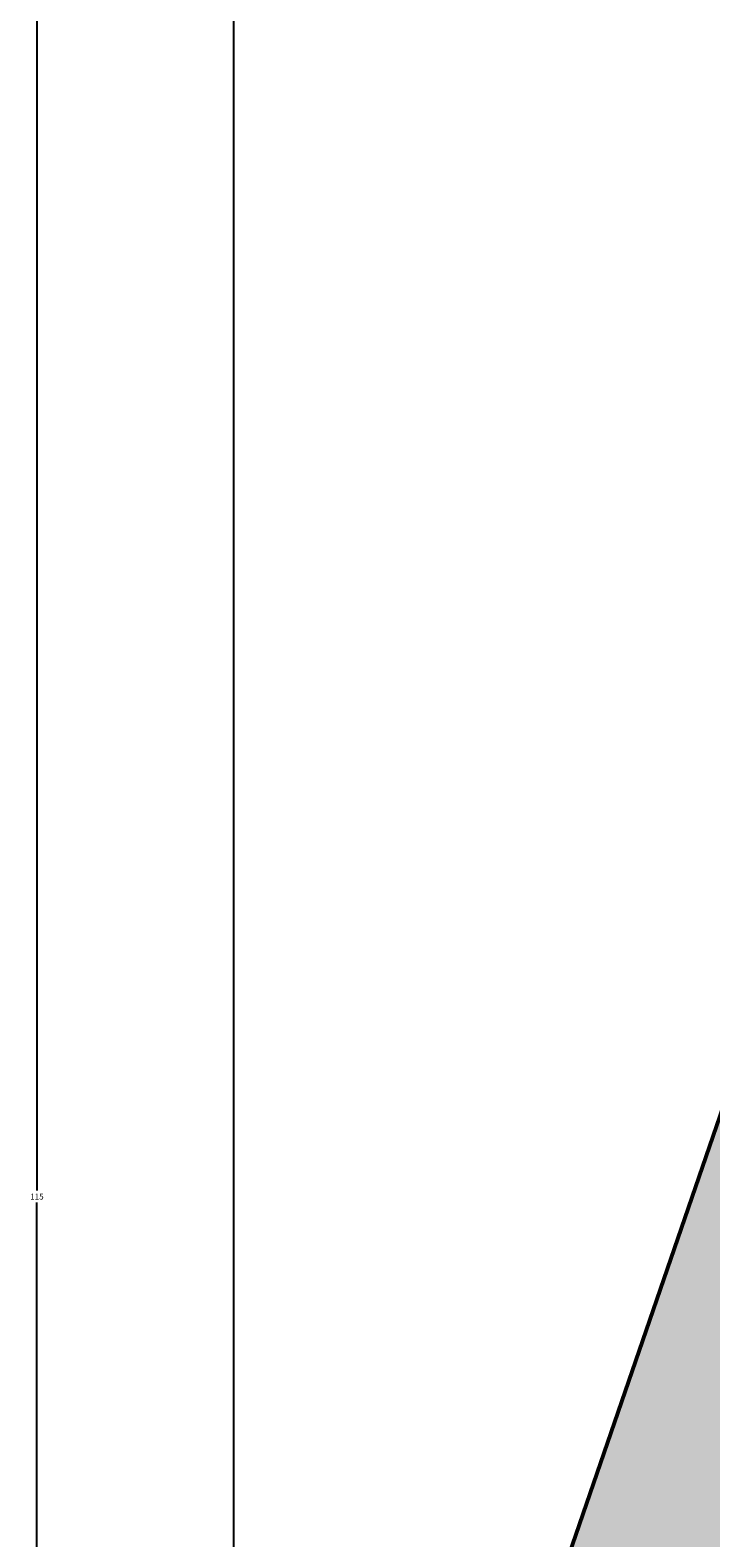
# Model space of a CAD drawing. Units: inches. Extents: x 114 to 236, y -51 to 115.
# Tile 5 of 14: x 114 to 135, y 41 to 87. Entities that reach past the tile are written whole.
import ezdxf

# ---------------------------------------------------------------- set-up
doc = ezdxf.new("R2010")
doc.units = ezdxf.units.IN
doc.header["$MEASUREMENT"] = 0
doc.layers.add('M-DIMS', color=2, linetype='Continuous', lineweight=18)
doc.layers.add('M-OUTL', color=7, linetype='Continuous', lineweight=50)
doc.layers.add('M-HATC', color=7, linetype='Continuous', lineweight=18, true_color=0xffffff)
doc.styles.get("Standard").update_dxf_attribs({"font": 'arial.ttf'})
doc.dimstyles.get("Standard").update_dxf_attribs({"dimtxt": 0.18, "dimasz": 0.18, "dimexe": 0.18, "dimexo": 0.0625, "dimgap": 0.09, "dimtad": 0, "dimtih": 1, "dimtoh": 1, "dimdec": 4, "dimzin": 0, "dimdsep": 46, "dimtxsty": 'Standard', "dimcen": 0.09, "dimadec": 0, "dimazin": 0, "dimtfac": 1, "dimtdec": 4, "dimtofl": 0, "dimtmove": 0, "dimatfit": 3, "dimfxl": 1, "dimtolj": 1, "dimtzin": 0, "dimarcsym": 0})

# ---------------------------------------------------------------- blocks, each defined once
blk = doc.blocks.new('*D3')
at = {"layer": 'Defpoints', "color": 0, "transparency": 16777216}
for p in [(230.229, 115.287), (120.229, 9.307), (230.229, 9.307)]:
    blk.add_point(p, dxfattribs=at)
at = {"layer": 'M-DIMS', "color": 0, "lineweight": -2, "transparency": 16777216}
for p, q in [((120.229, 9.37), (120.229, 115.467)), ((230.229, 9.37), (230.229, 115.467)), ((120.409, 115.287), (174.949, 115.287)), ((230.049, 115.287), (175.509, 115.287))]:
    blk.add_line(p, q, dxfattribs=at)
at = {"layer": 'M-DIMS', "color": 0, "transparency": 16777216}
for points in [[(120.409, 115.317), (120.409, 115.257), (120.229, 115.287)], [(230.049, 115.317), (230.049, 115.257), (230.229, 115.287)]]:
    blk.add_solid(points, dxfattribs=at)
at = {"layer": 'M-DIMS', "color": 0, "transparency": 16777216, "insert": (175.229, 115.287), "char_height": 0.18, "attachment_point": 5}
blk.add_mtext('\\A1;110', dxfattribs=at)
blk = doc.blocks.new('*D4')
at = {"layer": 'Defpoints', "color": 0, "transparency": 16777216}
for p in [(114.249, 109.307), (175.229, 109.307), (135.229, -5.693)]:
    blk.add_point(p, dxfattribs=at)
at = {"layer": 'M-DIMS', "color": 0, "lineweight": -2, "transparency": 16777216}
for p, q in [((175.166, 109.307), (114.069, 109.307)), ((114.249, 109.127), (114.249, 51.989)), ((114.249, -5.513), (114.249, 51.625)), ((135.166, -5.693), (114.069, -5.693))]:
    blk.add_line(p, q, dxfattribs=at)
at = {"layer": 'M-DIMS', "color": 0, "transparency": 16777216}
for points in [[(114.219, 109.127), (114.279, 109.127), (114.249, 109.307)], [(114.219, -5.513), (114.279, -5.513), (114.249, -5.693)]]:
    blk.add_solid(points, dxfattribs=at)
at = {"layer": 'M-DIMS', "color": 0, "transparency": 16777216, "insert": (114.249, 51.807), "char_height": 0.18, "attachment_point": 5}
blk.add_mtext('\\A1;115', dxfattribs=at)

msp = doc.modelspace()

# ---------------------------------------------------------------- hatches: boundary and pattern name
at = {"layer": 'M-HATC'}
h = msp.add_hatch(color=256, dxfattribs=at)
h.set_gradient(color1=(242, 103, 34), color2=(255, 255, 0), tint=1, name='INVSPHERICAL')
h.paths.add_polyline_path([(145.229, 79.307, -0.060651), (146.105, 86.505), (121.823, 16.038, -0.790743), (150.229, 9.307, -0.236068), (144.229, -2.693, -0.14094), (175.229, 9.098, -0.14094), (206.229, -2.693, -0.236068), (200.229, 9.307, -0.790743), (228.634, 16.038), (204.352, 86.505, -0.060651), (205.229, 79.307, -1)])

# ---------------------------------------------------------------- linework, layer by layer
at = {"layer": 'M-OUTL'}
msp.add_line((120.523, 12.263), (147.853, 91.577), dxfattribs=at)

# ---------------------------------------------------------------- dimensions: what is measured, and where the dimension line sits
at = {"layer": 'M-DIMS'}
dim = msp.add_linear_dim(base=(230.229, 115.287), p1=(120.229, 9.307), p2=(230.229, 9.307), dimstyle='Standard', override={"dimdec": 0, "dimlfac": 1, "dimrnd": 0, "dimzin": 0, "dimdsep": 46, "dimlunit": 2}, dxfattribs=at)
dim.commit()
dim.dimension.update_dxf_attribs({"geometry": '*D3', "text_midpoint": (175.229, 115.287)})
dim = msp.add_linear_dim(base=(114.249, 109.307), p1=(135.229, -5.693), p2=(175.229, 109.307), angle=90, dimstyle='Standard', override={"dimdec": 0, "dimlfac": 1, "dimrnd": 0, "dimzin": 0, "dimdsep": 46, "dimlunit": 2}, dxfattribs=at)
dim.commit()
dim.dimension.update_dxf_attribs({"geometry": '*D4', "text_midpoint": (114.249, 51.807)})

doc.saveas('drawing.dxf')
